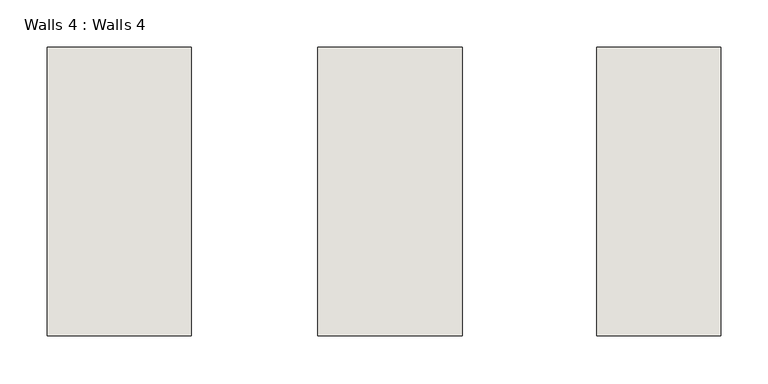
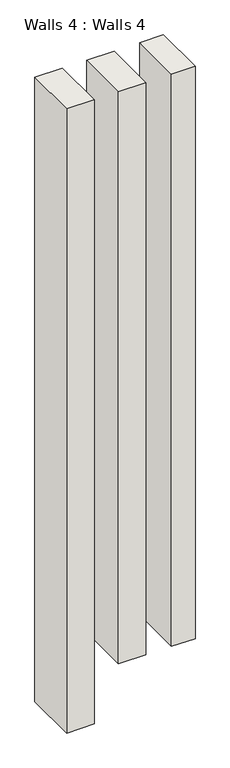
"""IFC4 building model written with IfcOpenShell, lengths in millimetres: wall geometry, Walls 4 : Walls 4."""

from ifc_helpers import new_model, si_unit, frame, origin, place, context, project, spatial, polyline, outline, extrude, source, transform, mapped, element, save


def walls_4_walls_4_19af3613(model_context):
    return source(origin(), model_context, "Body", "SweptSolid", [
        extrude(outline(polyline([(-15030.8766603, 3639.673096), (-15183.2766603, 3639.673096), (-15183.2766603, 3944.473096), (-15030.8766603, 3944.473096), (-15030.8766603, 3639.673096)])), frame((0.0, 0.0, 3962.4), z_axis=(0.0, 0.0, 1.0), x_axis=(1.0, 0.0, 0.0)), (0.0, 0.0, 1.0), 3657.6),
        extrude(outline(polyline([(-14744.7362863, 3639.673096), (-14897.1362863, 3639.673096), (-14897.1362863, 3944.473096), (-14744.7362863, 3944.473096), (-14744.7362863, 3639.673096)])), frame((0.0, 0.0, 4267.2), z_axis=(0.0, 0.0, 1.0), x_axis=(1.0, 0.0, 0.0)), (0.0, 0.0, 1.0), 3352.8),
        extrude(outline(polyline([(-14471.4087114, 3639.673096), (-14602.4968469, 3639.673096), (-14602.4968469, 3944.473096), (-14471.4087114, 3944.473096), (-14471.4087114, 3639.673096)])), frame((0.0, 0.0, 4267.2), z_axis=(0.0, 0.0, 1.0), x_axis=(1.0, 0.0, 0.0)), (0.0, 0.0, 1.0), 3352.8),
    ])


if __name__ == "__main__":
    model = new_model("IFC4")
    model_context = context("Model", 3, world=origin())
    ifc_project = project(units=[si_unit("LENGTHUNIT", "METRE", prefix="MILLI")], contexts=[model_context])
    site = spatial("IfcSite", under=ifc_project)
    building = spatial("IfcBuilding", under=site)
    placement = place(None, origin())
    walls_4_walls_4_shape = walls_4_walls_4_19af3613(model_context)
    element("IfcWall", 1, ObjectType="Walls 4 : Walls 4", at=placement, inside=building, context=model_context, shape_type="MappedRepresentation", body=[
        mapped(walls_4_walls_4_shape, transform((0.0, 0.0, 0.0), x_axis=(1.0, 0.0, 0.0), y_axis=(0.0, 1.0, 0.0), z_axis=(0.0, 0.0, 1.0))),
    ])
    save(model, "model.ifc")

# Revit data of these elements
# Element 1 (IfcWall, "Walls 4 : Walls 4")
#   Materials on its faces: "Default Wall"
# Materials
#   "Default Wall": colour RGB 128 128 128, transparency 0
